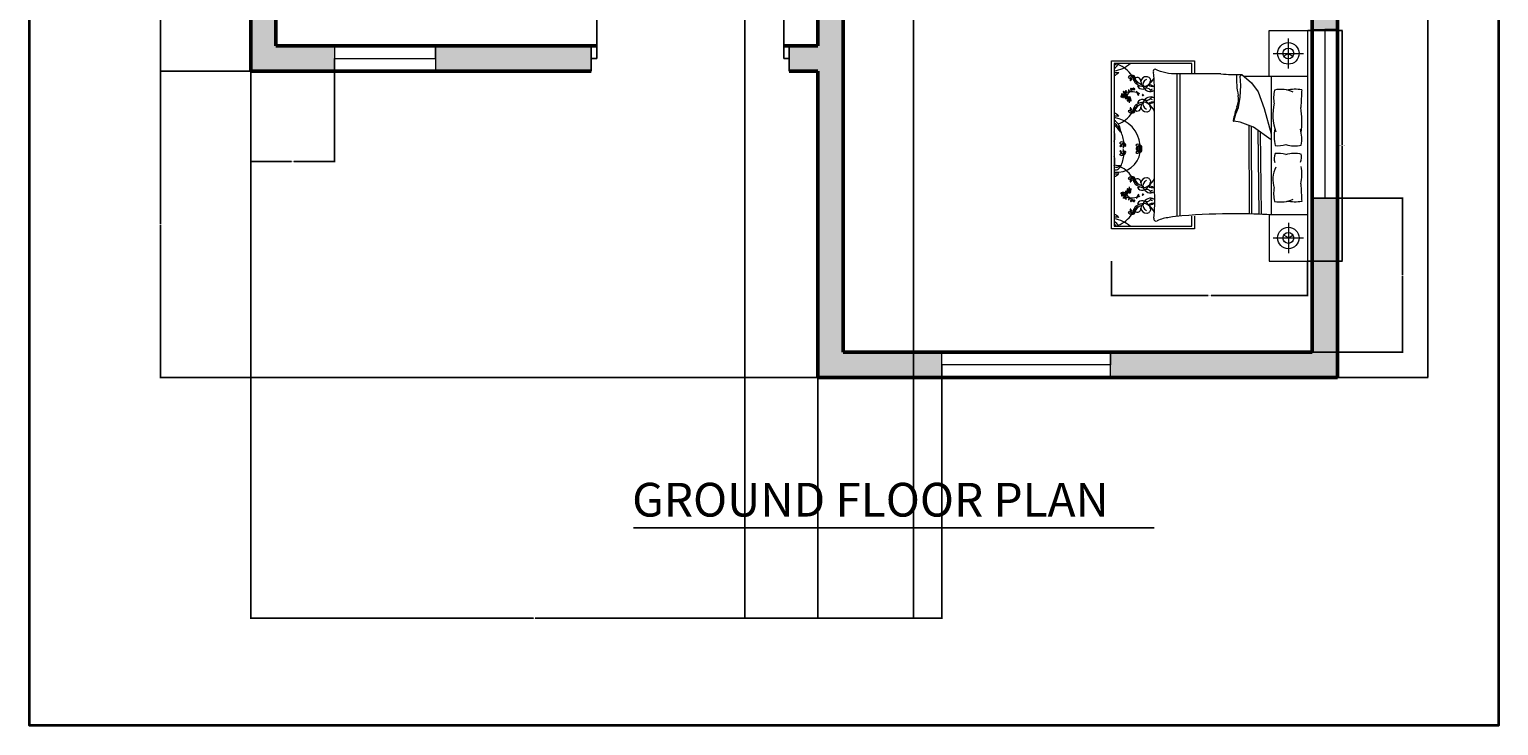
# Model space of a CAD drawing. Units: inches. Extents: x 1676 to 2199, y 1657 to 2783.
# Tile 1 of 10: x 1676 to 2199, y 1657 to 1905. Entities that reach past the tile are written whole.
import ezdxf

# ---------------------------------------------------------------- set-up
doc = ezdxf.new("R2010")
doc.units = ezdxf.units.IN
for name, color, linetype, lineweight in [('A-ANNO-DIMS', 2, 'Continuous', 18), ('A-ANNO-TEXT', 7, 'Continuous', 25), ('A-ANNO-TTLB', 7, 'Continuous', 35), ('A-DOOR', 4, 'Continuous', 25), ('A-FURN', 8, 'Continuous', 13), ('A-GLAZ', 4, 'Continuous', 18), ('A-WALL', 7, 'Continuous', 50)]:
    doc.layers.add(name, color=color, linetype=linetype, lineweight=lineweight)
doc.layers.add('A-WALL-PATT', color=251, linetype='Continuous', lineweight=13, true_color=0x636466)
doc.styles.get("Standard").update_dxf_attribs({"font": 'arial.ttf'})
doc.dimstyles.get("Standard").update_dxf_attribs({"dimtxt": 0.18, "dimasz": 0.18, "dimexe": 0.18, "dimexo": 0.0625, "dimgap": 0.09, "dimtad": 0, "dimtih": 1, "dimtoh": 1, "dimdec": 4, "dimzin": 0, "dimdsep": 46, "dimtxsty": 'Standard', "dimcen": 0.09, "dimadec": 0, "dimazin": 0, "dimtfac": 1, "dimtdec": 4, "dimtofl": 0, "dimtmove": 0, "dimatfit": 3, "dimfxl": 1, "dimtolj": 1, "dimtzin": 0, "dimarcsym": 0})

# ---------------------------------------------------------------- blocks, each defined once
blk = doc.blocks.new('BED-DOUBLE-WITH-NIGHTSTANDS')
for p, q in [((0, 0), (0, -82.08)), ((-6.84, -13.57), (-6.84, -2.85)), ((-12.2, -8.21), (-1.48, -8.21)), ((-69.81, -10.83), (-40.24, -10.83)), ((-69.81, -70.68), (-69.81, -10.83)), ((-68.85, -11.79), (-68.85, -69.72)), ((-41.19, -11.79), (-68.85, -11.79)), ((-46.38, -66.12), (-46.38, -15.47)), ((-45.36, -66.04), (-45.36, -15.47)), ((-41.19, -15.48), (-41.19, -11.79)), ((-40.24, -10.83), (-40.24, -15.48)), ((-24.05, -16.35), (-23.39, -15.68)), ((-23.39, -15.68), (-19.9, -18.67)), ((-60.53, -19.87), (-59.61, -19.69)), ((-23.72, -19.67), (-24.05, -16.35)), ((-24.05, -23.83), (-23.72, -19.67)), ((0, -16.42), (-22.53, -16.42)), ((-19.9, -18.67), (-17.57, -21.83)), ((-12.97, -16.42), (-12.97, -65.67)), ((-60.53, -25.61), (-59.61, -25.79)), ((-54.44, -57.71), (-54.44, -24.38)), ((-24.55, -27.49), (-24.05, -23.83)), ((-17.57, -21.83), (-15.41, -27.82)), ((-26.21, -32.31), (-25.55, -29.65)), ((-25.55, -29.65), (-24.55, -27.49)), ((-15.41, -27.82), (-12.97, -36.77)), ((-24.05, -32.64), (-26.21, -32.31)), ((-19.23, -34.47), (-24.05, -32.64)), ((-20.65, -65.38), (-20.78, -33.88)), ((-19.81, -65.37), (-19.93, -34.2)), ((-12.97, -38.97), (-19.23, -34.47)), ((-17.22, -65.41), (-17.64, -35.61)), ((-16.38, -65.45), (-16.79, -36.22)), ((-60.53, -55.9), (-59.61, -55.72)), ((-60.53, -61.64), (-59.61, -61.82)), ((-41.19, -69.72), (-41.19, -66.11)), ((-40.24, -66.12), (-40.24, -70.68)), ((-40.24, -70.68), (-69.81, -70.68)), ((-68.85, -69.72), (-41.19, -69.72)), ((-6.84, -68.51), (-6.84, -79.24)), ((-12.2, -73.87), (-1.48, -73.87))]:
    blk.add_line(p, q)
for points in [[(-13.68, -16.42), (-13.68, 0), (0, 0)], [(-6.84, -8.21), (-8.5, -9.17)], [(-6.84, -8.21), (-5.18, -9.17)], [(0, -65.67), (-13.68, -65.67), (-13.68, -82.08), (0, -82.08)], [(-6.84, -73.87), (-8.5, -72.92)], [(-6.84, -73.87), (-5.18, -72.92)]]:
    blk.add_lwpolyline(points)
for points in [[(-30.9, -15.51, 0.001242), (-46.48, -15.47, -0.127202), (-54.24, -13.83)], [(-2.05, -21.13, 0.074897), (-7.41, -21.23, -0.472817)], [(-7.71, -40.66, 0.14099), (-2.24, -40.82, 0.235245)], [(-7.71, -44.16, -0.14099), (-2.24, -44, -0.235245)], [(-2.05, -60.95, -0.074897), (-7.41, -60.85, 0.472817)], [(-44.71, -66.02, 0.056112), (-49.23, -66.61, 0.095341), (-53.58, -67.77)]]:
    blk.add_lwpolyline(points, format="xyb")
for centre, radius in [((-6.84, -8.21), 3.83), ((-6.84, -8.21), 1.92), ((-65.71, -23.25), 0.209), ((-63.51, -24.62), 0.209), ((-63.51, -56.89), 0.209), ((-65.71, -58.26), 0.209), ((-6.84, -73.87), 3.83), ((-6.84, -73.87), 1.92)]:
    blk.add_circle(centre, radius)
for centre, radius, start, end in [((-72.71, -7.3), 6.51, 306.3036, 316.4814), ((-71.73, -9.18), 5.22, 303.4617, 330.1116), ((-70.3, -3.81), 10.72, 277.745, 311.8856), ((-70.53, -12.11), 4.36, 292.5547, 318.9546), ((-68.18, -0.17), 14.83, 267.4081, 273.6519), ((-71.36, -22.14), 10.72, 34.3865, 68.5908), ((-54.19, -14.58), 0.757, 93.98, 207.3412), ((-139.89, -23.4), 85.45, 359.3433, 5.6887), ((-25.43, 59.58), 75.29, 265.8294, 271.553), ((-62.77, -17.25), 1.19, 77.7115, 159.0387), ((-63.41, -16.06), 0.895, 238.4633, 358.2869), ((-60.47, -17.87), 2.71, 138.8402, 177.9352), ((-63.05, -17.78), 0.133, 177.9352, 11.4834), ((-62.98, -17.77), 0.0647, 11.4834, 127.9409), ((-62.86, -20.88), 0.16, 142.4737, 265.053), ((-62.65, -20.85), 0.345, 127.7621, 169.0403), ((-62.11, -16.87), 0.877, 117.6827, 223.7762), ((-62.84, -20.56), 0.486, 265.053, 338.3618), ((-62.66, -17.39), 0.116, 223.7762, 159.7183), ((-62.19, -21.22), 0.635, 113.4276, 137.6104), ((-62.3, -16.95), 0.889, 2.9516, 103.728), ((-55.19, -14.46), 7.5, 192.5173, 207.1824), ((-63.5, -17.46), 1.69, 345.4653, 54.2343), ((-60.95, -15.14), 1.83, 211.3827, 255.2969), ((-62.27, -20.56), 0.209, 183.2768, 356.7232), ((-62.11, -20.94), 0.342, 139.7889, 227.6792), ((-62.92, -20.94), 0.684, 353.0852, 15.7171), ((-62.47, -21.02), 0.432, 350.3487, 43.6538), ((-61.67, -20.57), 0.503, 198.7263, 262.5032), ((-62.07, -20.81), 0.2, 1.1081, 91.8675), ((-60.23, -17.7), 1.54, 175.969, 254.3045), ((-60.6, -18), 1.23, 350.264, 160.8688), ((-61.94, -20.85), 0.349, 11.5637, 52.6358), ((-61.69, -20.92), 0.162, 255.2356, 54.9248), ((-61.93, -17.74), 0.755, 333.9755, 53.2681), ((-62.27, -19.36), 1.64, 6.1662, 51.5825), ((-57.89, -15.55), 3.88, 211.2614, 251.7045), ((-58.2, -15.52), 4.4, 236.2883, 266.5076), ((-58.76, -18.86), 2.04, 209.9085, 343.1337), ((-57.44, -18.45), 1.96, 84.9449, 172.8857), ((-57, -18.11), 2.38, 182.3591, 234.0401), ((-56.7, -19.22), 1.9, 111.5819, 201.4221), ((-58.27, -17.45), 2.47, 265.2933, 346.921), ((-57.91, -20.15), 0.509, 167.3041, 285.1471), ((-56.53, -22.59), 3.17, 122.7011, 126.3445), ((-55.93, -19.17), 2.62, 199.2822, 299.1751), ((-57.33, -22.26), 1.68, 41.5653, 105.1471), ((-57.24, -17.88), 1.39, 354.4856, 91.0538), ((-55.05, -16.54), 3.4, 238.8218, 279.1554), ((-56.53, -22.59), 3.17, 55.785, 94.7304), ((-60.22, -14.26), 6.21, 303.6671, 333.2997), ((-56.41, -18.78), 2.36, 277.436, 299.9149), ((-55.35, -20.75), 0.989, 30.0293, 52.325), ((5.68, -17.09), 30.98, 177.4519, 191.3392), ((-66.31, -23.57), 0.16, 142.4737, 265.053), ((-66.1, -23.53), 0.345, 61.2196, 169.0403), ((-66.28, -23.24), 0.486, 265.053, 338.3618), ((-65.87, -22.82), 0.413, 157.4086, 261.4386), ((-66.1, -22.81), 0.207, 58.0499, 135.6268), ((-65.64, -23.91), 0.635, 113.4276, 137.6104), ((-65.89, -22.94), 0.138, 172.906, 277.132), ((-66.34, -23.19), 0.659, 14.7558, 58.0499), ((-65.56, -23.63), 0.342, 139.7889, 227.6792), ((-65.67, -23.75), 0.18, 227.6792, 350.3487), ((-65.42, -23.02), 0.285, 36.1046, 181.4281), ((-66.36, -23.62), 0.684, 353.0852, 15.7171), ((-65.41, -21.9), 0.233, 124.3538, 214.3923), ((-65.06, -21.94), 0.544, 190.3057, 287.1958), ((-65.91, -23.7), 0.432, 350.3487, 43.6538), ((-65.59, -22.79), 0.288, 270.0645, 331.1507), ((-65.34, -22.86), 0.329, 221.8413, 265.7877), ((-65.11, -23.26), 0.503, 198.7263, 262.5032), ((-64.91, -21.74), 0.632, 176.9701, 248.2913), ((-60.4, -18.41), 6.11, 212.6784, 216.3746), ((-65.51, -23.49), 0.2, 1.1081, 91.8675), ((-65.34, -22.99), 0.205, 263.7526, 41.7054), ((-65.39, -23.54), 0.349, 11.5637, 86.365), ((-65.12, -21.89), 0.242, 216.3746, 291.7548), ((-62.98, -25.28), 3.41, 124.0033, 132.4917), ((-65.14, -23.6), 0.162, 255.2356, 54.9248), ((-66.49, -25.71), 3.64, 63.7819, 68.2913), ((-64.54, -22.91), 0.579, 128.3208, 208.8162), ((-64.54, -22.06), 0.544, 122.8155, 187.3992), ((-64.44, -22.87), 0.692, 207.7043, 254.3516), ((-64.96, -22.28), 0.182, 289.3605, 111.7548), ((-64.83, -22.28), 0.182, 221.8703, 44.2646), ((-64, -22.81), 0.953, 157.2305, 229.0635), ((-64.3, -22.13), 0.632, 109.4799, 177.6828), ((-64.32, -22.5), 0.561, 174.4544, 220.6188), ((-64.89, -23.26), 0.953, 270.278, 342.111), ((-64.25, -24.45), 0.674, 98.7227, 159.3375), ((-64.59, -23.59), 0.692, 244.9899, 291.6373), ((-67.51, -25.63), 4.09, 30.544, 49.818), ((-64.64, -21.73), 0.233, 56.8636, 146.9021), ((-64.52, -21.99), 0.242, 148.8844, 224.2646), ((-65.26, -23.3), 0.674, 340.0041, 40.6188), ((-59.5, -25.02), 6.11, 145.1882, 148.8844), ((-62.98, -25.28), 3.41, 94.756, 119.2041), ((-55.72, -30.19), 11.22, 132.2412, 142.1744), ((-64.44, -23.23), 0.561, 278.7227, 324.8872), ((-64.54, -23.69), 0.579, 290.5253, 358.5375), ((-64.11, -24.93), 0.16, 142.4737, 265.053), ((-63.89, -24.9), 0.345, 61.2196, 169.0403), ((-64.08, -24.61), 0.486, 265.053, 338.3618), ((-63.67, -24.19), 0.413, 157.4086, 261.4386), ((-63.9, -24.18), 0.207, 58.0499, 135.6268), ((-63.41, -23.52), 0.579, 182.8499, 266.1226), ((-63.63, -23.12), 0.561, 231.7607, 277.9252), ((-63.2, -23.02), 0.953, 214.5369, 286.3699), ((-63.43, -25.27), 0.635, 113.4276, 137.6104), ((-63.68, -24.31), 0.138, 172.906, 277.132), ((-64.14, -24.56), 0.659, 14.7558, 58.0499), ((-67.51, -25.63), 4.09, 23.0501, 23.8477), ((-61.39, -21.26), 2.31, 178.3264, 187.1302), ((-63.89, -21.58), 0.431, 11.3256, 64.4621), ((-62.42, -20.96), 1.3, 190.2588, 210.656), ((-63.35, -24.99), 0.342, 139.7889, 227.6792), ((-63.29, -21.49), 0.394, 188.3432, 274.2869), ((-63.46, -25.11), 0.18, 227.6792, 350.3487), ((-63.46, -24.34), 0.674, 37.3105, 97.9252), ((-62.95, -21.27), 0.688, 210.656, 242.6341), ((-63.22, -24.39), 0.285, 36.1046, 181.4281), ((-64.16, -24.99), 0.684, 353.0852, 15.7171), ((-62.43, -20.68), 1.32, 218.2101, 226.3071), ((-63.39, -23.41), 0.692, 265.0106, 311.658), ((-67.51, -25.63), 4.09, 357.1071, 4.7585), ((-63.71, -25.07), 0.432, 350.3487, 43.6538), ((-62.91, -24.63), 0.503, 198.7263, 262.5032), ((-63.38, -24.16), 0.288, 270.0645, 331.1507), ((-63.14, -24.23), 0.329, 221.8413, 265.7877), ((-63.4, -21.79), 0.167, 325.7657, 67.4417), ((-63.31, -24.86), 0.2, 1.1081, 91.8675), ((-68.6, -16.2), 7.79, 313.1541, 322.0459), ((-62.81, -28.67), 6.8, 73.5842, 93.8277), ((-63.14, -24.35), 0.205, 263.7526, 41.7054), ((-63.18, -24.91), 0.349, 11.5637, 86.365), ((-62.93, -24.97), 0.162, 255.2356, 54.9248), ((-62.22, -21.06), 0.18, 227.6792, 350.3487), ((-58.62, -21.75), 2.31, 178.3264, 187.1302), ((-61.12, -22.07), 0.431, 11.3256, 64.4621), ((-59.66, -21.45), 1.3, 190.2588, 210.656), ((-60.53, -21.98), 0.394, 188.3432, 274.2869), ((-60.19, -21.76), 0.688, 210.656, 242.6341), ((-59.67, -21.17), 1.32, 218.2101, 226.3071), ((-58.2, -29.97), 4.4, 93.4924, 123.7117), ((-60.64, -22.28), 0.167, 325.7657, 67.4417), ((-60.17, -22.58), 0.394, 147.5332, 233.4768), ((-58.76, -26.63), 2.04, 16.8663, 150.0915), ((-59.81, -22.38), 0.688, 179.1859, 211.164), ((-60.49, -22.54), 0.167, 354.3784, 96.0543), ((-62.81, -28.67), 6.8, 63.0032, 69.8941), ((-59.29, -22.07), 1.3, 211.164, 231.5612), ((-59.07, -21.01), 2.31, 234.6898, 243.4936), ((-59.05, -22.2), 1.32, 195.5129, 203.6099), ((-60.53, -23.06), 0.431, 357.3579, 50.4944), ((-57, -27.38), 2.38, 125.9599, 177.6409), ((-58.68, -22.98), 0.158, 12.7051, 190.4384), ((-58.58, -22.96), 0.257, 190.4384, 10.4136), ((-56.7, -26.27), 1.9, 158.5779, 248.4181), ((-58.27, -28.03), 2.47, 13.079, 94.7067), ((-57.91, -25.34), 0.509, 74.8529, 192.6959), ((-55.93, -26.31), 2.62, 60.8249, 160.7178), ((-56.53, -22.9), 3.17, 233.6555, 237.2989), ((-57.33, -23.22), 1.68, 254.8529, 318.4347), ((-55.05, -28.95), 3.4, 79.7133, 121.1782), ((-56.53, -22.9), 3.17, 265.2696, 304.215), ((-60.22, -31.22), 6.21, 21.4941, 56.3329), ((-56.41, -26.71), 2.36, 60.0851, 82.564), ((-55.16, -20.33), 1.23, 221.5653, 293.8354), ((-55.16, -25.15), 1.23, 66.1646, 138.4347), ((-55.35, -24.73), 0.989, 307.675, 336.7144), ((-55.35, -20.75), 0.989, 314.4517, 333.558), ((-55.35, -24.73), 0.989, 23.229, 45.5483), ((-31.24, -24.49), 6.68, 336.2616, 11.3392), ((6.73, -29.85), 19.08, 168.0397, 199.2615), ((-1.09, -24.06), 11, 165.1039, 191.0369), ((-9.56, -31.59), 10.58, 65.1316, 101.7583), ((779.11, -66.37), 782.47, 176.68521, 177.14978), ((-70.53, -33.38), 4.36, 41.0454, 67.4453), ((-68.18, -45.32), 14.83, 86.3481, 92.5919), ((-70.3, -41.68), 10.72, 4.4623, 82.255), ((-71.36, -23.34), 10.72, 291.4092, 325.6135), ((-63.41, -29.42), 0.895, 1.7131, 121.5367), ((-62.77, -28.23), 1.19, 200.9613, 282.2885), ((-63.05, -27.7), 0.133, 348.5166, 182.0648), ((-60.47, -27.61), 2.71, 182.0648, 221.1598), ((-62.98, -27.72), 0.0647, 232.0591, 348.5166), ((-62.11, -28.62), 0.877, 136.2238, 242.3173), ((-62.61, -28.1), 0.0699, 200.2667, 136.2271), ((-63.5, -28.02), 1.69, 305.7657, 14.5347), ((-55.19, -31.02), 7.5, 152.8176, 167.4827), ((-62.3, -28.53), 0.889, 256.272, 357.0484), ((-60.95, -30.35), 1.83, 104.7031, 148.6173), ((-60.23, -27.78), 1.54, 105.6955, 184.031), ((-60.6, -27.49), 1.23, 199.1312, 9.736), ((-61.93, -27.74), 0.755, 306.7319, 26.0245), ((-62.27, -26.13), 1.64, 308.4175, 353.8338), ((-57.89, -29.93), 3.88, 108.2955, 148.7386), ((-57.44, -27.04), 1.96, 187.1143, 275.0551), ((-57.24, -27.61), 1.39, 268.9462, 5.5144), ((4.81, -38.01), 31.83, 160.1194, 169.3383), ((-31.75, -32.38), 29.77, 352.2196, 9.497), ((-71.73, -36.3), 5.22, 1.272, 56.5383), ((-72.71, -38.18), 6.51, 17.8504, 53.6964), ((-74.54, -41.6), 9.68, 34.0123, 54.053), ((-74.49, -37.86), 5.89, 343.5431, 17.0202), ((-76.04, -40.86), 10.72, 4.4623, 27.4146), ((-26.28, -32.12), 0.198, 178.8623, 289.7536), ((2.57, -37.57), 14.48, 169.8617, 193.6238), ((-16.7, -38.67), 14.63, 351.5249, 13.96), ((-77.53, -40.2), 8.72, 4.3787, 5.6357), ((-83.5, -44.79), 15.58, 19.7217, 19.9028), ((-66.15, -40.91), 1.19, 47.7873, 129.1145), ((-66.12, -39.56), 0.895, 208.5391, 328.3627), ((-66.66, -41.22), 0.133, 148.011, 341.5592), ((-64.48, -42.59), 2.71, 108.9159, 148.011), ((-66.6, -41.25), 0.0647, 341.5592, 98.0167), ((-65.39, -40.9), 0.877, 87.7585, 193.852), ((-66.13, -41.08), 0.116, 193.852, 129.9245), ((-58.2, -42.27), 7.5, 162.593, 177.2582), ((-66.9, -40.72), 1.69, 315.5411, 24.3101), ((-63.52, -39.98), 1.83, 181.4585, 225.3727), ((-65.6, -40.88), 0.889, 333.0274, 73.8037), ((-60.41, -41.73), 1.19, 47.7873, 129.1145), ((-60.38, -40.38), 0.895, 208.5391, 328.3627), ((-58.73, -43.41), 2.71, 108.9159, 148.011), ((-59.65, -41.72), 0.877, 87.7585, 193.852), ((-60.39, -41.9), 0.116, 193.852, 129.9245), ((-61.16, -41.54), 1.69, 315.5411, 24.3101), ((-52.46, -43.09), 7.5, 162.593, 177.2582), ((-61.16, -42.7), 1.69, 335.6899, 44.4589), ((-52.46, -41.16), 7.5, 182.7418, 197.407), ((-59.86, -41.7), 0.889, 333.0274, 73.8037), ((-57.78, -40.8), 1.83, 181.4585, 225.3727), ((-10.45, -30.98), 10.06, 264.0129, 285.8293), ((-67.82, -42.22), 8.3, 262.8636, 351.8197), ((-74.49, -46.39), 5.89, 342.9798, 16.4569), ((-77.53, -44.05), 8.72, 354.3643, 355.6213), ((-83.5, -39.46), 15.58, 340.0972, 340.2783), ((-66.12, -44.69), 0.895, 31.6373, 151.4609), ((-66.15, -43.34), 1.19, 230.8855, 312.2127), ((-66.66, -43.02), 0.133, 18.4408, 211.989), ((-64.48, -41.66), 2.71, 211.989, 251.0841), ((-66.6, -43), 0.0647, 261.9833, 18.4408), ((-76.04, -43.39), 10.72, 332.5854, 355.5377), ((-65.39, -43.35), 0.877, 166.148, 272.2415), ((-66.08, -43.15), 0.0699, 230.1909, 166.0209), ((-58.2, -41.98), 7.5, 182.7418, 197.407), ((-66.9, -43.52), 1.69, 335.6899, 44.4589), ((-63.52, -44.27), 1.83, 134.6273, 178.5415), ((-65.6, -43.37), 0.889, 286.1963, 26.9726), ((-60.38, -43.87), 0.895, 31.6373, 151.4609), ((-60.41, -42.52), 1.19, 230.8855, 312.2127), ((-60.92, -42.04), 0.133, 148.011, 341.5592), ((-60.92, -42.2), 0.133, 18.4408, 211.989), ((-58.73, -40.84), 2.71, 211.989, 251.0841), ((-60.86, -42.07), 0.0647, 341.5592, 98.0167), ((-60.86, -42.18), 0.0647, 261.9833, 18.4408), ((-59.65, -42.52), 0.877, 166.148, 272.2415), ((-60.34, -42.33), 0.0699, 230.1909, 166.0209), ((-59.86, -42.55), 0.889, 286.1963, 26.9726), ((-57.78, -43.45), 1.83, 134.6273, 178.5415), ((-7.56, -45.67), 4.35, 155.0183, 198.5407), ((-10.45, -53.84), 10.06, 74.1707, 95.9871), ((-6.14, -45.12), 4.06, 333.3437, 16.1026), ((-67.07, -43.29), 4.8, 248.117, 276.6195), ((-68.4, -47.7), 1.92, 256.3898, 349.0739), ((-68.14, -46.25), 2.43, 252.8609, 311.9049), ((-68.18, -36.19), 14.83, 267.4081, 273.6519), ((-70.53, -48.13), 4.36, 292.5547, 318.9546), ((-71.36, -58.17), 10.72, 34.3865, 68.5908), ((-62.77, -53.28), 1.19, 77.7115, 159.0387), ((-63.41, -52.09), 0.895, 238.4633, 358.2869), ((-60.47, -53.9), 2.71, 138.8402, 177.9352), ((-62.11, -52.89), 0.877, 117.6827, 223.7762), ((-62.3, -52.98), 0.889, 2.9516, 103.728), ((-60.95, -51.16), 1.83, 211.3827, 255.2969), ((-63.5, -53.49), 1.69, 345.4653, 54.2343), ((-55.19, -50.49), 7.5, 192.5173, 207.1824), ((-1.9, -53.28), 10.45, 153.8761, 196.1746), ((-16.41, -51.21), 14.43, 346.3427, 11.1841), ((-64.59, -57.92), 0.692, 68.3627, 115.0101), ((-64.89, -58.25), 0.953, 17.889, 89.722), ((-64.25, -57.06), 0.674, 200.6625, 261.2773), ((-64.54, -57.82), 0.579, 1.4625, 69.4747), ((-64.11, -56.58), 0.16, 94.947, 217.5263), ((-63.89, -56.61), 0.345, 190.9597, 298.7804), ((-64.08, -56.9), 0.486, 21.6382, 94.947), ((-63.67, -57.32), 0.413, 98.5614, 202.5914), ((-63.9, -57.33), 0.207, 224.3732, 301.9501), ((-63.41, -57.99), 0.579, 93.8774, 177.1501), ((-63.2, -58.49), 0.953, 73.6301, 145.4631), ((-63.43, -56.24), 0.635, 222.3896, 246.5724), ((-63.68, -57.2), 0.138, 82.868, 187.094), ((-64.14, -56.95), 0.659, 301.9501, 345.2442), ((-67.51, -55.88), 4.09, 336.1523, 336.9499), ((-63.35, -56.52), 0.342, 132.3208, 220.2111), ((-63.46, -56.4), 0.18, 9.6513, 132.3208), ((-64.16, -56.52), 0.684, 344.2829, 6.9148), ((-63.22, -57.12), 0.285, 178.5719, 323.8954), ((-63.39, -58.1), 0.692, 48.342, 94.9894), ((-67.51, -55.88), 4.09, 355.2415, 2.8929), ((-63.71, -56.44), 0.432, 316.3462, 9.6513), ((-62.91, -56.88), 0.503, 97.4968, 161.2737), ((-63.14, -57.28), 0.329, 94.2123, 138.1587), ((-63.38, -57.35), 0.288, 28.8493, 89.9355), ((-63.31, -56.65), 0.2, 268.1325, 358.8919), ((-63.05, -53.81), 0.133, 177.9352, 11.4834), ((-63.18, -56.6), 0.349, 273.635, 348.4363), ((-63.14, -57.16), 0.205, 318.2946, 96.2474), ((-62.98, -53.79), 0.0647, 11.4834, 127.9409), ((-62.93, -56.54), 0.162, 305.0752, 104.7644), ((-62.66, -53.42), 0.116, 223.7762, 159.7183), ((-60.23, -53.73), 1.54, 175.969, 254.3045), ((-60.6, -54.02), 1.23, 350.264, 160.8688), ((-61.93, -53.77), 0.755, 333.9755, 53.2681), ((-62.27, -55.38), 1.64, 6.1662, 51.5825), ((-57.89, -51.58), 3.88, 211.2614, 251.7045), ((-58.2, -51.54), 4.4, 236.2883, 266.5076), ((-58.76, -54.88), 2.04, 209.9085, 343.1337), ((-57.44, -54.47), 1.96, 84.9449, 172.8857), ((-57, -54.13), 2.38, 182.3591, 234.0401), ((-56.7, -55.24), 1.9, 111.5819, 201.4221), ((-58.27, -53.48), 2.47, 265.2933, 346.921), ((-57.91, -56.17), 0.509, 167.3041, 285.1471), ((-56.53, -58.61), 3.17, 122.7011, 126.3445), ((-55.93, -55.2), 2.62, 199.2822, 299.1751), ((-57.33, -58.29), 1.68, 41.5653, 105.1471), ((-57.24, -53.9), 1.39, 354.4856, 91.0538), ((-55.05, -52.56), 3.4, 238.8218, 280.2867), ((-56.53, -58.61), 3.17, 55.785, 94.7304), ((-60.22, -50.29), 6.21, 303.6671, 338.5059), ((-56.41, -54.8), 2.36, 277.436, 299.9149), ((-55.16, -56.36), 1.23, 221.5653, 293.8354), ((-55.35, -56.78), 0.989, 23.2856, 52.325), ((-55.35, -56.78), 0.989, 314.4517, 336.7144), ((-1.09, -58.02), 11, 168.9631, 194.8961), ((779.11, -15.71), 782.47, 182.85022, 183.31479), ((-66.31, -57.94), 0.16, 94.947, 217.5263), ((-66.1, -57.98), 0.345, 190.9597, 298.7804), ((-66.28, -58.27), 0.486, 21.6382, 94.947), ((-65.87, -58.69), 0.413, 98.5614, 202.5914), ((-66.1, -58.7), 0.207, 224.3732, 301.9501), ((-65.64, -57.6), 0.635, 222.3896, 246.5724), ((-65.89, -58.57), 0.138, 82.868, 187.094), ((-66.34, -58.32), 0.659, 301.9501, 345.2442), ((-65.56, -57.88), 0.342, 132.3208, 220.2111), ((-65.67, -57.76), 0.18, 9.6513, 132.3208), ((-66.36, -57.89), 0.684, 344.2829, 6.9148), ((-65.42, -58.49), 0.285, 178.5719, 323.8954), ((-65.41, -59.61), 0.233, 145.6077, 235.6462), ((-65.91, -57.81), 0.432, 316.3462, 9.6513), ((-65.06, -59.58), 0.544, 72.8042, 169.6943), ((-65.11, -58.25), 0.503, 97.4968, 161.2737), ((-65.34, -58.65), 0.329, 94.2123, 138.1587), ((-65.59, -58.72), 0.288, 28.8493, 89.9355), ((-64.91, -59.77), 0.632, 111.7087, 183.0299), ((-60.4, -63.1), 6.11, 143.6254, 147.3216), ((-65.51, -58.02), 0.2, 268.1325, 358.8919), ((-65.39, -57.97), 0.349, 273.635, 348.4363), ((-65.34, -58.52), 0.205, 318.2946, 96.2474), ((-65.12, -59.62), 0.242, 68.2452, 143.6254), ((-62.98, -56.23), 3.41, 227.5083, 235.9967), ((-65.14, -57.91), 0.162, 305.0752, 104.7644), ((-66.49, -55.8), 3.64, 291.7087, 296.2181), ((-64.54, -58.6), 0.579, 151.1838, 231.6792), ((-64.54, -59.45), 0.544, 172.6008, 237.1845), ((-64.44, -58.64), 0.692, 105.6484, 152.2957), ((-64.96, -59.23), 0.182, 248.2452, 70.6395), ((-64.83, -59.23), 0.182, 315.7354, 138.1297), ((-64, -58.7), 0.953, 130.9365, 202.7695), ((-64.3, -59.38), 0.632, 182.3172, 250.5201), ((-64.32, -59.01), 0.561, 139.3812, 185.5456), ((-67.51, -55.88), 4.09, 310.182, 329.456), ((-64.64, -59.78), 0.233, 213.0979, 303.1364), ((-64.52, -59.52), 0.242, 135.7354, 211.1156), ((-65.26, -58.21), 0.674, 319.3812, 19.9959), ((-59.5, -56.49), 6.11, 211.1156, 214.8118), ((-62.98, -56.23), 3.41, 240.7959, 265.244), ((-55.72, -51.32), 11.22, 217.8256, 227.7588), ((-64.44, -58.28), 0.561, 35.1128, 81.2773), ((-63.63, -58.39), 0.561, 82.0748, 128.2393), ((-62.42, -60.55), 1.3, 149.344, 169.7412), ((-61.39, -60.25), 2.31, 172.8698, 181.6736), ((-63.89, -59.93), 0.431, 295.5379, 348.6744), ((-63.29, -60.02), 0.394, 85.7131, 171.6568), ((-63.46, -57.17), 0.674, 262.0748, 322.6895), ((-62.95, -60.24), 0.688, 117.3659, 149.344), ((-62.43, -60.83), 1.32, 133.6929, 141.7899), ((-63.4, -59.72), 0.167, 292.5583, 34.2343), ((-62.81, -52.84), 6.8, 266.1723, 286.4158), ((-68.6, -65.31), 7.79, 37.9541, 46.8459), ((-62.86, -60.63), 0.16, 94.947, 217.5263), ((-62.65, -60.66), 0.345, 190.9597, 232.2379), ((-62.84, -60.95), 0.486, 21.6382, 94.947), ((-62.19, -60.29), 0.635, 222.3896, 246.5724), ((-62.27, -60.95), 0.209, 3.2768, 176.7232), ((-62.11, -60.57), 0.342, 132.3208, 220.2111), ((-62.22, -60.45), 0.18, 9.6513, 132.3208), ((-62.92, -60.57), 0.684, 344.2829, 6.9148), ((-62.47, -60.49), 0.432, 316.3462, 9.6513), ((-61.67, -60.94), 0.503, 97.4968, 161.2737), ((-62.07, -60.7), 0.2, 268.1325, 358.8919), ((-60.23, -63.81), 1.54, 105.6955, 184.031), ((-61.69, -60.6), 0.162, 305.0752, 104.7644), ((-61.94, -60.66), 0.349, 307.3642, 348.4363), ((-62.27, -62.15), 1.64, 308.4175, 353.8338), ((-57.89, -65.96), 3.88, 108.2955, 148.7386), ((-59.66, -60.06), 1.3, 149.344, 169.7412), ((-58.62, -59.76), 2.31, 172.8698, 181.6736), ((-61.12, -59.44), 0.431, 295.5379, 348.6744), ((-60.53, -59.53), 0.394, 85.7131, 171.6568), ((-60.19, -59.75), 0.688, 117.3659, 149.344), ((-59.67, -60.34), 1.32, 133.6929, 141.7899), ((-58.2, -65.99), 4.4, 93.4924, 123.7117), ((-60.64, -59.23), 0.167, 292.5583, 34.2343), ((-60.17, -58.93), 0.394, 126.5232, 212.4668), ((-58.76, -62.65), 2.04, 16.8663, 150.0915), ((-59.81, -59.13), 0.688, 148.836, 180.8141), ((-60.49, -58.97), 0.167, 263.9457, 5.6216), ((-62.81, -52.84), 6.8, 290.1059, 296.9968), ((-59.29, -59.44), 1.3, 128.4388, 148.836), ((-59.07, -60.5), 2.31, 116.5064, 125.3102), ((-59.05, -59.31), 1.32, 156.3901, 164.4871), ((-60.53, -58.45), 0.431, 309.5056, 2.6421), ((-57, -63.4), 2.38, 125.9599, 177.6409), ((-58.68, -58.53), 0.158, 169.5616, 347.2949), ((-58.58, -58.55), 0.257, 349.5864, 169.5616), ((-56.7, -62.29), 1.9, 158.5779, 248.4181), ((-58.27, -64.06), 2.47, 13.079, 94.7067), ((-57.91, -61.36), 0.509, 74.8529, 192.6959), ((-55.93, -62.34), 2.62, 60.8249, 160.7178), ((-56.53, -58.92), 3.17, 233.6555, 237.2989), ((-57.33, -59.25), 1.68, 254.8529, 318.4347), ((-55.05, -64.97), 3.4, 79.249, 121.1782), ((-56.53, -58.92), 3.17, 265.2696, 304.215), ((-60.22, -67.25), 6.21, 23.6453, 56.3329), ((-56.41, -62.73), 2.36, 60.0851, 82.564), ((-55.16, -61.18), 1.23, 66.1646, 138.4347), ((-55.35, -60.76), 0.989, 307.675, 342.5814), ((-134.28, -60.22), 79.87, 355.2402, 1.8035), ((-55.35, -60.76), 0.989, 16.6343, 45.5483), ((-9.56, -50.49), 10.58, 258.2417, 294.8684), ((-70.53, -69.4), 4.36, 41.0454, 67.4453), ((-68.18, -81.34), 14.83, 86.3481, 92.5919), ((-70.3, -77.7), 10.72, 48.1144, 82.255), ((-71.73, -72.33), 5.22, 29.8884, 56.5383), ((-71.36, -59.37), 10.72, 291.4092, 325.6135), ((-63.41, -65.45), 0.895, 1.7131, 121.5367), ((-62.77, -64.26), 1.19, 200.9613, 282.2885), ((-63.05, -63.73), 0.133, 348.5166, 182.0648), ((-60.47, -63.64), 2.71, 182.0648, 221.1598), ((-62.98, -63.74), 0.0647, 232.0591, 348.5166), ((-62.11, -64.64), 0.877, 136.2238, 242.3173), ((-62.61, -64.13), 0.0699, 200.2667, 136.2271), ((-55.19, -67.05), 7.5, 152.8176, 167.4827), ((-63.5, -64.05), 1.69, 305.7657, 14.5347), ((-60.95, -66.37), 1.83, 104.7031, 148.6173), ((-62.3, -64.56), 0.889, 256.272, 357.0484), ((-60.6, -63.51), 1.23, 199.1312, 9.736), ((-61.93, -63.77), 0.755, 306.7319, 26.0245), ((-57.44, -63.06), 1.96, 187.1143, 275.0551), ((-57.24, -63.63), 1.39, 268.9462, 5.5144), ((-53.99, -67.14), 0.748, 156.5219, 303.8264), ((-28.37, -257.71), 192.39, 89.1145, 94.8735), ((-23, -212.81), 147.49, 86.1, 90.9282), ((-72.71, -74.21), 6.51, 43.5186, 53.6964)]:
    blk.add_arc(centre, radius, start, end)
blk = doc.blocks.new('WIN-60')
for p, q in [((0, 0), (9, 0)), ((9, 0), (4.5, 0)), ((4.5, 0), (4.5, -60)), ((4.5, -60), (0, -60)), ((0, -60), (9, -60))]:
    blk.add_line(p, q)
blk = doc.blocks.new('*D11')
at = {"layer": 'A-ANNO-DIMS', "color": 0, "lineweight": -2, "transparency": 16777216}
for p, q in [((2131.47, 1904.65), (2143.9, 1904.65)), ((2143.72, 1904.47), (2143.72, 1863.8)), ((2143.72, 1822.75), (2143.72, 1863.43)), ((2131.47, 1822.57), (2143.9, 1822.57))]:
    blk.add_line(p, q, dxfattribs=at)
at = {"layer": 'A-ANNO-DIMS', "color": 0, "transparency": 16777216}
for points in [[(2143.69, 1904.47), (2143.75, 1904.47), (2143.72, 1904.65)], [(2143.69, 1822.75), (2143.75, 1822.75), (2143.72, 1822.57)]]:
    blk.add_solid(points, dxfattribs=at)
at = {"layer": 'Defpoints', "color": 0, "transparency": 16777216}
for p in [(2131.41, 1904.65), (2143.72, 1904.65), (2131.41, 1822.57)]:
    blk.add_point(p, dxfattribs=at)
at = {"layer": 'A-ANNO-DIMS', "color": 0, "transparency": 16777216, "insert": (2143.72, 1863.61), "char_height": 0.18, "attachment_point": 5}
blk.add_mtext('\\A1;BED GROUP 82 TYP.', dxfattribs=at)
blk = doc.blocks.new('*D12')
at = {"layer": 'A-ANNO-DIMS', "color": 0, "lineweight": -2, "transparency": 16777216}
for p, q in [((2061.6, 1822.51), (2061.6, 1810.08)), ((2131.41, 1822.51), (2131.41, 1810.08)), ((2061.78, 1810.26), (2095.98, 1810.26)), ((2131.23, 1810.26), (2097.03, 1810.26))]:
    blk.add_line(p, q, dxfattribs=at)
at = {"layer": 'A-ANNO-DIMS', "color": 0, "transparency": 16777216}
for points in [[(2061.78, 1810.29), (2061.78, 1810.23), (2061.6, 1810.26)], [(2131.23, 1810.29), (2131.23, 1810.23), (2131.41, 1810.26)]]:
    blk.add_solid(points, dxfattribs=at)
at = {"layer": 'Defpoints', "color": 0, "transparency": 16777216}
for p in [(2061.6, 1822.57), (2131.41, 1822.57), (2131.41, 1810.26)]:
    blk.add_point(p, dxfattribs=at)
at = {"layer": 'A-ANNO-DIMS', "color": 0, "transparency": 16777216, "insert": (2096.51, 1810.26), "char_height": 0.18, "attachment_point": 5}
blk.add_mtext('\\A1;70 TYP.', dxfattribs=at)
blk = doc.blocks.new('*D20')
at = {"layer": 'A-ANNO-DIMS', "color": 0, "lineweight": -2, "transparency": 16777216}
for p, q in [((2142.14, 2341.09), (2174.4, 2341.09)), ((2174.22, 2340.91), (2174.22, 2061.27)), ((2174.22, 1781.27), (2174.22, 2060.91)), ((2142.14, 1781.09), (2174.4, 1781.09))]:
    blk.add_line(p, q, dxfattribs=at)
at = {"layer": 'A-ANNO-DIMS', "color": 0, "transparency": 16777216}
for points in [[(2174.19, 2340.91), (2174.25, 2340.91), (2174.22, 2341.09)], [(2174.19, 1781.27), (2174.25, 1781.27), (2174.22, 1781.09)]]:
    blk.add_solid(points, dxfattribs=at)
at = {"layer": 'Defpoints', "color": 0, "transparency": 16777216}
for p in [(2142.07, 2341.09), (2174.22, 2341.09), (2142.07, 1781.09)]:
    blk.add_point(p, dxfattribs=at)
at = {"layer": 'A-ANNO-DIMS', "color": 0, "transparency": 16777216, "insert": (2174.22, 2061.09), "char_height": 0.18, "attachment_point": 5}
blk.add_mtext('\\A1;560', dxfattribs=at)
blk = doc.blocks.new('*D21')
at = {"layer": 'A-ANNO-DIMS', "color": 0, "lineweight": -2, "transparency": 16777216}
for p, q in [((1755.07, 1890.02), (1755.07, 1695.28)), ((1957.07, 1781.02), (1957.07, 1695.28)), ((1755.25, 1695.46), (1855.79, 1695.46)), ((1956.89, 1695.46), (1856.36, 1695.46))]:
    blk.add_line(p, q, dxfattribs=at)
at = {"layer": 'A-ANNO-DIMS', "color": 0, "transparency": 16777216}
for points in [[(1755.25, 1695.49), (1755.25, 1695.43), (1755.07, 1695.46)], [(1956.89, 1695.49), (1956.89, 1695.43), (1957.07, 1695.46)]]:
    blk.add_solid(points, dxfattribs=at)
at = {"layer": 'Defpoints', "color": 0, "transparency": 16777216}
for p in [(1755.07, 1890.09), (1957.07, 1781.09), (1957.07, 1695.46)]:
    blk.add_point(p, dxfattribs=at)
at = {"layer": 'A-ANNO-DIMS', "color": 0, "transparency": 16777216, "insert": (1856.07, 1695.46), "char_height": 0.18, "attachment_point": 5}
blk.add_mtext('\\A1;202', dxfattribs=at)
blk = doc.blocks.new('*D22')
at = {"layer": 'A-ANNO-DIMS', "color": 0, "lineweight": -2, "transparency": 16777216}
for p, q in [((1755.07, 1890.02), (1755.07, 1857.76)), ((1784.92, 1890.02), (1784.92, 1857.76)), ((1755.25, 1857.94), (1769.6, 1857.94)), ((1784.74, 1857.94), (1770.4, 1857.94))]:
    blk.add_line(p, q, dxfattribs=at)
at = {"layer": 'A-ANNO-DIMS', "color": 0, "transparency": 16777216}
for points in [[(1755.25, 1857.97), (1755.25, 1857.91), (1755.07, 1857.94)], [(1784.74, 1857.97), (1784.74, 1857.91), (1784.92, 1857.94)]]:
    blk.add_solid(points, dxfattribs=at)
at = {"layer": 'Defpoints', "color": 0, "transparency": 16777216}
for p in [(1755.07, 1890.09), (1784.92, 1890.09), (1755.07, 1857.94)]:
    blk.add_point(p, dxfattribs=at)
at = {"layer": 'A-ANNO-DIMS', "color": 0, "transparency": 16777216, "insert": (1770, 1857.94), "char_height": 0.18, "attachment_point": 5}
blk.add_mtext('\\A1;29.85', dxfattribs=at)
blk = doc.blocks.new('*D23')
at = {"layer": 'A-ANNO-DIMS', "color": 0, "lineweight": -2, "transparency": 16777216}
for p, q in [((1957.07, 1781.02), (1957.07, 1695.28)), ((2001.21, 1781.02), (2001.21, 1695.28)), ((1957.25, 1695.46), (1978.68, 1695.46)), ((2001.03, 1695.46), (1979.61, 1695.46))]:
    blk.add_line(p, q, dxfattribs=at)
at = {"layer": 'A-ANNO-DIMS', "color": 0, "transparency": 16777216}
for points in [[(1957.25, 1695.49), (1957.25, 1695.43), (1957.07, 1695.46)], [(2001.03, 1695.49), (2001.03, 1695.43), (2001.21, 1695.46)]]:
    blk.add_solid(points, dxfattribs=at)
at = {"layer": 'Defpoints', "color": 0, "transparency": 16777216}
for p in [(1957.07, 1781.09), (2001.21, 1781.09), (2001.21, 1695.46)]:
    blk.add_point(p, dxfattribs=at)
at = {"layer": 'A-ANNO-DIMS', "color": 0, "transparency": 16777216, "insert": (1979.14, 1695.46), "char_height": 0.18, "attachment_point": 5}
blk.add_mtext('\\A1;44.136', dxfattribs=at)
blk = doc.blocks.new('*D24')
at = {"layer": 'A-ANNO-DIMS', "color": 0, "lineweight": -2, "transparency": 16777216}
for p, q in [((1755.01, 1890.09), (1722.74, 1890.09)), ((1722.92, 1889.91), (1722.92, 1835.77)), ((1722.92, 1781.27), (1722.92, 1835.41)), ((1957.01, 1781.09), (1722.74, 1781.09))]:
    blk.add_line(p, q, dxfattribs=at)
at = {"layer": 'A-ANNO-DIMS', "color": 0, "transparency": 16777216}
for points in [[(1722.89, 1889.91), (1722.95, 1889.91), (1722.92, 1890.09)], [(1722.89, 1781.27), (1722.95, 1781.27), (1722.92, 1781.09)]]:
    blk.add_solid(points, dxfattribs=at)
at = {"layer": 'Defpoints', "color": 0, "transparency": 16777216}
for p in [(1722.92, 1890.09), (1755.07, 1890.09), (1957.07, 1781.09)]:
    blk.add_point(p, dxfattribs=at)
at = {"layer": 'A-ANNO-DIMS', "color": 0, "transparency": 16777216, "insert": (1722.92, 1835.59), "char_height": 0.18, "attachment_point": 5}
blk.add_mtext('\\A1;109', dxfattribs=at)
blk = doc.blocks.new('*D25')
at = {"layer": 'A-ANNO-DIMS', "color": 0, "lineweight": -2, "transparency": 16777216}
for p, q in [((1755.01, 1959.57), (1722.74, 1959.57)), ((1722.92, 1959.39), (1722.92, 1925.01)), ((1722.92, 1890.27), (1722.92, 1924.65)), ((1755.01, 1890.09), (1722.74, 1890.09))]:
    blk.add_line(p, q, dxfattribs=at)
at = {"layer": 'A-ANNO-DIMS', "color": 0, "transparency": 16777216}
for points in [[(1722.89, 1959.39), (1722.95, 1959.39), (1722.92, 1959.57)], [(1722.89, 1890.27), (1722.95, 1890.27), (1722.92, 1890.09)]]:
    blk.add_solid(points, dxfattribs=at)
at = {"layer": 'Defpoints', "color": 0, "transparency": 16777216}
for p in [(1722.92, 1959.57), (1755.07, 1959.57), (1755.07, 1890.09)]:
    blk.add_point(p, dxfattribs=at)
at = {"layer": 'A-ANNO-DIMS', "color": 0, "transparency": 16777216, "insert": (1722.92, 1924.83), "char_height": 0.18, "attachment_point": 5}
blk.add_mtext('\\A1;69.49', dxfattribs=at)
blk = doc.blocks.new('*D30')
at = {"layer": 'A-ANNO-DIMS', "color": 0, "lineweight": -2, "transparency": 16777216}
for p, q in [((2133.14, 1844.99), (2165.4, 1844.99)), ((2165.22, 1844.81), (2165.22, 1817.72)), ((2165.22, 1790.27), (2165.22, 1817.36)), ((2133.14, 1790.09), (2165.4, 1790.09))]:
    blk.add_line(p, q, dxfattribs=at)
at = {"layer": 'A-ANNO-DIMS', "color": 0, "transparency": 16777216}
for points in [[(2165.19, 1844.81), (2165.25, 1844.81), (2165.22, 1844.99)], [(2165.19, 1790.27), (2165.25, 1790.27), (2165.22, 1790.09)]]:
    blk.add_solid(points, dxfattribs=at)
at = {"layer": 'Defpoints', "color": 0, "transparency": 16777216}
for p in [(2133.07, 1844.99), (2133.07, 1790.09), (2165.22, 1790.09)]:
    blk.add_point(p, dxfattribs=at)
at = {"layer": 'A-ANNO-DIMS', "color": 0, "transparency": 16777216, "insert": (2165.22, 1817.54), "char_height": 0.18, "attachment_point": 5}
blk.add_mtext('\\A1;54.9', dxfattribs=at)
blk = doc.blocks.new('*D40')
at = {"layer": 'A-ANNO-DIMS', "color": 0, "lineweight": -2, "transparency": 16777216}
for p, q in [((1931.07, 2236.02), (1931.07, 1695.28)), ((1991.07, 2236.02), (1991.07, 1695.28)), ((1931.25, 1695.46), (1960.86, 1695.46)), ((1990.89, 1695.46), (1961.29, 1695.46))]:
    blk.add_line(p, q, dxfattribs=at)
at = {"layer": 'A-ANNO-DIMS', "color": 0, "transparency": 16777216}
for points in [[(1931.25, 1695.49), (1931.25, 1695.43), (1931.07, 1695.46)], [(1990.89, 1695.49), (1990.89, 1695.43), (1991.07, 1695.46)]]:
    blk.add_solid(points, dxfattribs=at)
at = {"layer": 'Defpoints', "color": 0, "transparency": 16777216}
for p in [(1931.07, 2236.09), (1991.07, 2236.09), (1991.07, 1695.46)]:
    blk.add_point(p, dxfattribs=at)
at = {"layer": 'A-ANNO-DIMS', "color": 0, "transparency": 16777216, "insert": (1961.07, 1695.46), "char_height": 0.18, "attachment_point": 5}
blk.add_mtext('\\A1;60', dxfattribs=at)

msp = doc.modelspace()

# ---------------------------------------------------------------- hatches: boundary and pattern name
at = {"layer": 'A-WALL-PATT'}
h = msp.add_hatch(color=256, dxfattribs=at)
h.dxf.hatch_style = 1
h.paths.add_polyline_path([(1945.4216, 2336.5871), (1945.4216, 2341.0871), (1755.075, 2341.0871), (1755.075, 2323.0739), (1764.075, 2323.0739), (1764.075, 2332.0871), (1945.4216, 2332.0871)])
h.paths.add_polyline_path([(1764.075, 2299.0739), (1755.075, 2299.0739), (1755.075, 2266.2601), (1759.575, 2266.2601), (1764.075, 2266.2601)])
h.paths.add_polyline_path([(1843.075, 2285.0871), (1764.075, 2285.0871), (1764.075, 2276.0871), (1843.075, 2276.0871)])
h.paths.add_polyline_path([(1931.075, 2332.0871), (1922.075, 2332.0871), (1922.075, 2285.0871), (1907.247, 2285.0871), (1907.247, 2276.0871), (1922.075, 2276.0871), (1922.075, 2263.0871), (1922.075, 2214.434), (1922.075, 2183.2198), (1931.075, 2183.2198), (1931.075, 2214.434), (1931.075, 2227.0871), (1991.075, 2227.0871), (1991.075, 2176.0871), (1991.075, 2167.0871), (2000.075, 2167.0871), (2133.075, 2167.0871), (2133.075, 2176.0871), (2000.075, 2176.0871), (2000.075, 2245.3418), (1995.575, 2245.3418), (1991.075, 2245.3418), (1991.075, 2236.0871), (1931.075, 2236.0871)])
h.paths.add_polyline_path([(2000.075, 2332.0871), (1991.075, 2332.0871), (1991.075, 2285.0871), (1991.075, 2274.6339), (2000.075, 2274.6339), (2000.075, 2285.0871)], flags=17)
h.paths.add_polyline_path([(2142.075, 2341.0871), (1969.4216, 2341.0871), (1969.4216, 2332.0871), (2133.075, 2332.0871), (2133.075, 2298.2101), (2142.075, 2298.2101)])
h.paths.add_polyline_path([(2142.075, 1844.9908), (2133.075, 1844.9908), (2133.075, 1790.0871), (2061.2106, 1790.0871), (2061.2106, 1781.0871), (2142.075, 1781.0871)])
h.paths.add_polyline_path([(2001.2106, 1790.0871), (1966.075, 1790.0871), (1966.075, 1957.0871), (1973.4183, 1957.0871), (1973.4183, 1966.0871), (1966.075, 1966.0871), (1966.075, 1983.1515), (1957.075, 1983.1515), (1957.075, 1899.0871), (1946.8789, 1899.0871), (1946.8789, 1890.0871), (1957.075, 1890.0871), (1957.075, 1781.0871), (2001.2106, 1781.0871), (2001.2106, 1785.5871)])
h.paths.add_polyline_path([(1876.3163, 1894.5871), (1876.3163, 1899.0871), (1820.9237, 1899.0871), (1820.9237, 1890.0871), (1876.3163, 1890.0871)])
h.paths.add_polyline_path([(1764.075, 2093.9207), (1759.575, 2093.9207), (1755.075, 2093.9207), (1755.075, 2019.5723), (1764.075, 2019.5723)])
h.paths.add_polyline_path([(1878.3926, 2083.0871), (1764.075, 2083.0871), (1764.075, 2074.0871), (1878.3926, 2074.0871)])
h.paths.add_polyline_path([(1764.075, 1959.5723), (1755.075, 1959.5723), (1755.075, 1890.0871), (1784.9237, 1890.0871), (1784.9237, 1894.5871), (1784.9237, 1899.0871), (1764.075, 1899.0871)])
h.paths.add_polyline_path([(2133.075, 2047.0871), (2000.075, 2047.0871), (1966.075, 2047.0871), (1957.075, 2047.0871), (1938.4046, 2047.0871), (1938.4046, 2038.0871), (1957.075, 2038.0871), (1957.075, 2026.1604), (1966.075, 2026.1604), (1966.075, 2038.0871), (2039.075, 2038.0871), (2039.075, 2011.4216), (2048.075, 2011.4216), (2048.075, 2038.0871), (2133.075, 2038.0871)])
h.paths.add_polyline_path([(2133.075, 1966.0871), (2048.075, 1966.0871), (2048.075, 1972.5045), (2039.075, 1972.5045), (2039.075, 1966.0871), (2025.1075, 1966.0871), (2025.1075, 1957.0871), (2133.075, 1957.0871)])
h.paths.add_polyline_path([(1764.075, 2206.2601), (1755.075, 2206.2601), (1755.075, 2153.9207), (1764.075, 2153.9207)])
h = msp.add_hatch(color=256, dxfattribs=at)
h.dxf.hatch_style = 1
h.paths.add_polyline_path([(2142.075, 2238.2101), (2133.075, 2238.2101), (2133.075, 2023.2789), (2142.075, 2023.2789)])
h.paths.add_polyline_path([(2142.075, 1997.2789), (2133.075, 1997.2789), (2133.075, 1904.9908), (2142.075, 1904.9908)])

# ---------------------------------------------------------------- linework, layer by layer
at = {"layer": 'A-ANNO-TEXT'}
msp.add_line((1891.3582, 1727.6113), (2076.7522, 1727.6113), dxfattribs=at)
at = {"layer": 'A-ANNO-TTLB'}
msp.add_lwpolyline([(1676.2722, 2782.5054), (2199.4461, 2782.5054), (2199.4461, 1657.2705), (1676.2722, 1657.2705)], close=True, dxfattribs=at)
at = {"layer": 'A-DOOR'}
for p, q in [((1878.3163, 1894.5871), (1878.3163, 1942.5871)), ((1944.8789, 1894.5871), (1944.8789, 1942.5871)), ((1876.3163, 1899.0871), (1876.3163, 1890.0871)), ((1876.3163, 1890.0871), (1876.3163, 1894.5871)), ((1876.3163, 1894.5871), (1878.3163, 1894.5871)), ((1946.8789, 1894.5871), (1944.8789, 1894.5871)), ((1946.8789, 1890.0871), (1946.8789, 1899.0871))]:
    msp.add_line(p, q, dxfattribs=at)
at = {"layer": 'A-GLAZ'}
for p, q in [((1784.9237, 1899.0871), (1784.9237, 1890.0871)), ((1784.9237, 1890.0871), (1784.9237, 1894.5871)), ((1784.9237, 1894.5871), (1820.9237, 1894.5871)), ((1820.9237, 1894.5871), (1820.9237, 1899.0871)), ((1820.9237, 1899.0871), (1820.9237, 1890.0871))]:
    msp.add_line(p, q, dxfattribs=at)
at = {"layer": 'A-WALL'}
for p, q in [((1755.075, 2341.0871), (1755.075, 1890.0871)), ((2142.075, 2341.0871), (2142.075, 1781.0871)), ((1764.075, 2332.0871), (1764.075, 1899.0871)), ((2133.075, 2332.0871), (2133.075, 1790.0871)), ((1957.075, 1983.1515), (1957.075, 1899.0871)), ((1966.075, 1957.0871), (1966.075, 1790.0871)), ((1764.075, 1899.0871), (1878.3163, 1899.0871)), ((1944.8789, 1899.0871), (1957.075, 1899.0871)), ((1755.075, 1890.0871), (1876.3163, 1890.0871)), ((1946.8789, 1890.0871), (1957.075, 1890.0871)), ((1957.075, 1890.0871), (1957.075, 1781.0871)), ((1966.075, 1790.0871), (2133.075, 1790.0871)), ((1957.075, 1781.0871), (2142.075, 1781.0871))]:
    msp.add_line(p, q, dxfattribs=at)

# ---------------------------------------------------------------- block references
at = {"layer": 'A-FURN'}
msp.add_blockref('BED-DOUBLE-WITH-NIGHTSTANDS', (2131.4084, 1904.6541), dxfattribs=at)
at = {"layer": 'A-GLAZ'}
msp.add_blockref('WIN-60', (2133.075, 1904.9908), dxfattribs=at)
at = {"layer": 'A-GLAZ', "extrusion": (0, 0, -1), "zscale": -1, "rotation": 90}
msp.add_blockref('WIN-60', (-2061.2106, 1781.0871), dxfattribs=at)

# ---------------------------------------------------------------- texts
at = {"layer": 'A-ANNO-TEXT', "insert": (1890.9097, 1743.6493), "char_height": 12, "attachment_point": 1}
msp.add_mtext_dynamic_manual_height_columns('GROUND FLOOR PLAN', width=423.017701, gutter_width=12.5, heights=[0], dxfattribs=at)

# ---------------------------------------------------------------- dimensions: what is measured, and where the dimension line sits
at = {"layer": 'A-ANNO-DIMS'}
for base, p1, p2, angle, override, picture, middle in [((2174.225, 2341.0871), (2142.075, 1781.0871), (2142.075, 2341.0871), 90, {"dimdec": 0, "dimlfac": 1, "dimrnd": 0, "dimzin": 0, "dimdsep": 46, "dimlunit": 2}, '*D20', (2174.225, 2061.0871)), ((1722.925, 1959.5723), (1755.075, 1890.0871), (1755.075, 1959.5723), 90, {"dimdec": 2, "dimlfac": 1, "dimrnd": 0, "dimzin": 0, "dimdsep": 46, "dimlunit": 2}, '*D25', (1722.925, 1924.8297)), ((1722.925, 1890.0871), (1957.075, 1781.0871), (1755.075, 1890.0871), 90, {"dimdec": 0, "dimlfac": 1, "dimrnd": 0, "dimzin": 0, "dimdsep": 46, "dimlunit": 2}, '*D24', (1722.925, 1835.5871)), ((1755.075, 1857.9371), (1784.9237, 1890.0871), (1755.075, 1890.0871), 180, {"dimdec": 2, "dimlfac": 1, "dimrnd": 0, "dimzin": 0, "dimdsep": 46, "dimlunit": 2}, '*D22', (1769.9994, 1857.9371)), ((2165.225, 1790.0871), (2133.075, 1844.9908), (2133.075, 1790.0871), 270, {"dimdec": 1, "dimlfac": 1, "dimrnd": 0, "dimzin": 0, "dimdsep": 46, "dimlunit": 2}, '*D30', (2165.225, 1817.5389))]:
    dim = msp.add_linear_dim(base=base, p1=p1, p2=p2, angle=angle, dimstyle='Standard', override=override, dxfattribs=at)
    dim.commit()
    dim.dimension.update_dxf_attribs({"geometry": picture, "text_midpoint": middle})
for base, p1, p2, override, picture, middle in [((1991.075, 1695.4613), (1931.075, 2236.0871), (1991.075, 2236.0871), {"dimdec": 0, "dimlfac": 1, "dimrnd": 0, "dimzin": 0, "dimdsep": 46, "dimlunit": 2}, '*D40', (1961.075, 1695.4613)), ((1957.075, 1695.4613), (1755.075, 1890.0871), (1957.075, 1781.0871), {"dimdec": 0, "dimlfac": 1, "dimrnd": 0, "dimzin": 0, "dimdsep": 46, "dimlunit": 2}, '*D21', (1856.075, 1695.4613)), ((2001.2106, 1695.4613), (1957.075, 1781.0871), (2001.2106, 1781.0871), {"dimdec": 3, "dimlfac": 1, "dimrnd": 0, "dimzin": 0, "dimdsep": 46, "dimlunit": 2}, '*D23', (1979.1428, 1695.4613))]:
    dim = msp.add_linear_dim(base=base, p1=p1, p2=p2, dimstyle='Standard', override=override, dxfattribs=at)
    dim.commit()
    dim.dimension.update_dxf_attribs({"geometry": picture, "text_midpoint": middle})
dim = msp.add_linear_dim(base=(2143.7209, 1904.6541), p1=(2131.4084, 1822.5711), p2=(2131.4084, 1904.6541), angle=90, text='BED GROUP <> TYP.', dimstyle='Standard', override={"dimdec": 0, "dimlfac": 1, "dimrnd": 0, "dimzin": 0, "dimdsep": 46, "dimlunit": 2}, dxfattribs=at)
dim.commit()
dim.dimension.update_dxf_attribs({"geometry": '*D11', "text_midpoint": (2143.7209, 1863.6126)})
dim = msp.add_linear_dim(base=(2131.4084, 1810.2586), p1=(2061.6023, 1822.5711), p2=(2131.4084, 1822.5711), text='<> TYP.', dimstyle='Standard', override={"dimdec": 0, "dimlfac": 1, "dimrnd": 0, "dimzin": 0, "dimdsep": 46, "dimlunit": 2}, dxfattribs=at)
dim.commit()
dim.dimension.update_dxf_attribs({"geometry": '*D12', "text_midpoint": (2096.5054, 1810.2586)})

doc.saveas('drawing.dxf')
